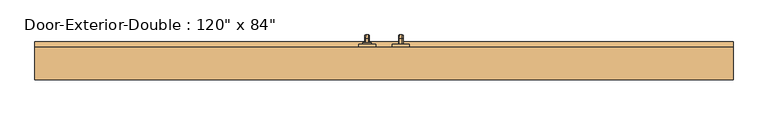
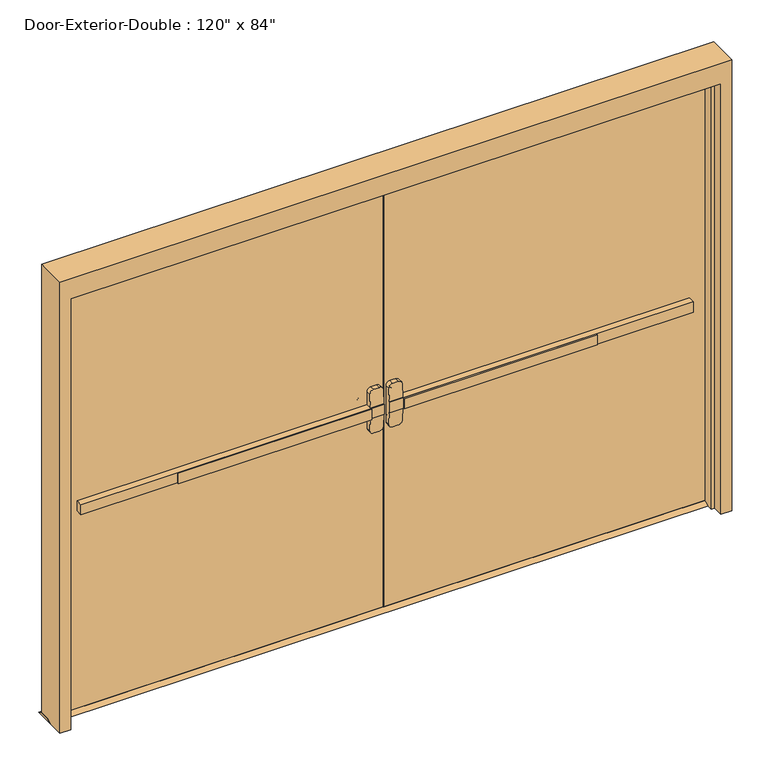
"""IFC4 building model written with IfcOpenShell, lengths in millimetres: door geometry."""

from ifc_helpers import new_model, si_unit, point, frame, frame_2d, origin, place, context, project, spatial, polyline, circle_curve, ellipse_curve, trimmed, segment, composite_curve, outline, extrude, faceted_brep, source, transform, mapped, element, save
from ifc_brep_helpers import plane_surface, cylinder_surface, revolved_surface, advanced_brep


def door_4e55e581(model_context):
    return source(origin(), model_context, "Body", "SolidModel", [
        extrude(outline(polyline([(-982.1333333, 0.0), (-982.1333333, 6.35), (-76.2, 6.35), (-76.2, 0.0), (-982.1333333, 0.0)])), frame((0.0, 0.0, 990.6), z_axis=(0.0, 0.0, 1.0), x_axis=(1.0, 0.0, 0.0)), (0.0, 0.0, 1.0), 50.8),
        advanced_brep(
        [(-12.7, 6.35, 1041.4), (-76.2, 6.35, 1041.4), (-1435.1, 6.35, 1041.4), (-1435.1, 6.35, 990.6), (-76.2, 6.35, 990.6), (-12.7, 6.35, 990.6), (-1435.1, 38.1, 1041.4), (-76.2, 38.1, 1041.4), (-76.2, 38.1, 1104.9), (-57.15, 38.1, 1123.95), (-31.75, 38.1, 1123.95), (-12.7, 38.1, 1104.9), (-12.7, 38.1, 927.1), (-31.75, 38.1, 908.05), (-57.15, 38.1, 908.05), (-76.2, 38.1, 927.1), (-76.2, 38.1, 990.6), (-1435.1, 38.1, 990.6), (-12.7, 9.5252467, 1041.4), (-76.2, 9.5252467, 1041.4), (-12.7, 9.5252467, 990.6), (-12.7, 14.5354269, 927.1), (-12.7, 14.5354269, 1104.9), (-76.2, 9.5252467, 990.6), (-76.2, 14.5354269, 1104.9), (-76.2, 14.5354269, 927.1), (-57.15, 16.038481, 1123.95), (-31.75, 16.038481, 1123.95), (-31.75, 16.038481, 908.05), (-57.15, 16.038481, 908.05)],
        [
            (0, 1),
            (1, 2),
            (2, 3),
            (3, 4),
            (4, 5),
            (5, 0),
            (6, 7),
            (7, 8),
            (8, 9, circle_curve(frame((-57.15, 38.1, 1104.9), z_axis=(0.0, 1.0, 0.0), x_axis=(-1.0, 0.0, 0.0)), 19.05)),
            (9, 10),
            (10, 11, circle_curve(frame((-31.75, 38.1, 1104.9), z_axis=(0.0, 1.0, 0.0), x_axis=(-1.0, 0.0, 0.0)), 19.05)),
            (11, 12),
            (12, 13, circle_curve(frame((-31.75, 38.1, 927.1), z_axis=(0.0, 1.0, 0.0), x_axis=(-1.0, 0.0, 0.0)), 19.05)),
            (13, 14),
            (14, 15, circle_curve(frame((-57.15, 38.1, 927.1), z_axis=(0.0, 1.0, 0.0), x_axis=(-1.0, 0.0, 0.0)), 19.05)),
            (15, 16),
            (16, 17),
            (17, 6),
            (0, 18),
            (18, 19),
            (19, 7),
            (6, 2),
            (5, 20),
            (20, 21),
            (21, 12),
            (11, 22),
            (22, 18),
            (16, 23),
            (23, 20),
            (3, 17),
            (19, 24),
            (24, 8),
            (15, 25),
            (25, 23),
            (9, 26),
            (26, 27),
            (27, 10),
            (13, 28),
            (28, 29),
            (29, 14),
            (29, 25, ellipse_curve(frame((-57.15, 14.5354269, 927.1), z_axis=(0.0, 0.9969018152893365, 0.07865602756830282), x_axis=(0.0, -0.07865602756830208, 0.9969018152893365)), 19.1092038, 19.05)),
            (24, 26, ellipse_curve(frame((-57.15, 14.5354269, 1104.9), z_axis=(0.0, 0.9969018152893376, -0.07865602756828934), x_axis=(0.0, -0.078656027568288, -0.9969018152893377)), 19.1092038, 19.05)),
            (27, 22, ellipse_curve(frame((-31.75, 14.5354269, 1104.9), z_axis=(0.0, 0.9969018152893376, -0.07865602756828934), x_axis=(0.0, -0.078656027568288, -0.9969018152893377)), 19.1092038, 19.05)),
            (21, 28, ellipse_curve(frame((-31.75, 14.5354269, 927.1), z_axis=(0.0, 0.9969018152893365, 0.07865602756830282), x_axis=(0.0, -0.07865602756830208, 0.9969018152893365)), 19.1092038, 19.05)),
        ],
        [
            plane_surface(frame((-12.7, 6.35, 1041.4), z_axis=(0.0, -1.0, 0.0), x_axis=(1.0, 0.0, 0.0))),
            plane_surface(frame((-12.7, 38.1, 1041.4), z_axis=(0.0, 1.0, 0.0), x_axis=(-1.0, 0.0, 0.0))),
            plane_surface(frame((-1435.1, 6.35, 1041.4), z_axis=(0.0, 0.0, 1.0), x_axis=(0.0, 1.0, 0.0))),
            plane_surface(frame((-12.7, 6.35, 1041.4), z_axis=(1.0, 0.0, 0.0), x_axis=(0.0, 1.0, 0.0))),
            plane_surface(frame((-12.7, 6.35, 990.6), z_axis=(0.0, 0.0, -1.0), x_axis=(0.0, 1.0, 0.0))),
            plane_surface(frame((-1435.1, 6.35, 990.6), z_axis=(-1.0, 0.0, 0.0), x_axis=(0.0, 1.0, 0.0))),
            plane_surface(frame((-76.2, 9.5252467, 927.1), z_axis=(-1.0, 0.0, 0.0), x_axis=(0.0, 1.0, 0.0))),
            plane_surface(frame((-57.15, 9.5252467, 1123.95), z_axis=(0.0, 0.0, 1.0), x_axis=(0.0, 1.0, 0.0))),
            plane_surface(frame((-31.75, 9.5252467, 908.05), z_axis=(0.0, 0.0, -1.0), x_axis=(0.0, 1.0, 0.0))),
            cylinder_surface(frame((-57.15, 38.1, 927.1), z_axis=(0.0, -1.0, 0.0), x_axis=(-1.0, 0.0, 0.0)), 19.05),
            cylinder_surface(frame((-57.15, 38.1, 1104.9), z_axis=(0.0, -1.0, 0.0), x_axis=(-1.0, 0.0, 0.0)), 19.05),
            cylinder_surface(frame((-31.75, 38.1, 1104.9), z_axis=(0.0, -1.0, 0.0), x_axis=(-1.0, 0.0, 0.0)), 19.05),
            cylinder_surface(frame((-31.75, 38.1, 927.1), z_axis=(0.0, -1.0, 0.0), x_axis=(-1.0, 0.0, 0.0)), 19.05),
            plane_surface(frame((-76.2, 9.5252467, 1041.4), z_axis=(0.0, -0.9969018152893376, 0.07865602756828934), x_axis=(1.0, 0.0, 0.0))),
            plane_surface(frame((-76.2, 16.038481, 908.05), z_axis=(0.0, -0.9969018152893365, -0.07865602756830282), x_axis=(1.0, 0.0, 0.0))),
        ],
        [
            (0, [[1, 2, 3, 4, 5, 6]]),
            (1, [[7, 8, 9, 10, 11, 12, 13, 14, 15, 16, 17, 18]]),
            (2, [[-2, -1, 19, 20, 21, -7, 22]]),
            (3, [[23, 24, 25, -12, 26, 27, -19, -6]]),
            (4, [[-17, 28, 29, -23, -5, -4, 30]]),
            (5, [[-22, -18, -30, -3]]),
            (6, [[-21, 31, 32, -8]]),
            (6, [[33, 34, -28, -16]]),
            (7, [[35, 36, 37, -10]]),
            (8, [[38, 39, 40, -14]]),
            (9, [[-40, 41, -33, -15]]),
            (10, [[-32, 42, -35, -9]]),
            (11, [[-37, 43, -26, -11]]),
            (12, [[-25, 44, -38, -13]]),
            (13, [[-27, -43, -36, -42, -31, -20]]),
            (14, [[-29, -34, -41, -39, -44, -24]]),
        ],
    ),
        extrude(outline(polyline([(82.55, 12.7), (107.95, 0.0), (12.7, 0.0), (38.1, 12.7), (82.55, 12.7)])), frame((-1574.8, 0.0, 0.0), z_axis=(1.0, 0.0, 0.0), x_axis=(0.0, 1.0, 0.0)), (0.0, 0.0, 1.0), 3149.6),
        extrude(outline(polyline([(982.1333333, 0.0), (76.2, 0.0), (76.2, 6.35), (982.1333333, 6.35), (982.1333333, 0.0)])), frame((0.0, 0.0, 990.6), z_axis=(0.0, 0.0, 1.0), x_axis=(1.0, 0.0, 0.0)), (0.0, 0.0, 1.0), 50.8),
        advanced_brep(
        [(12.7, 6.35, 1041.4), (12.7, 6.35, 990.6), (76.2, 6.35, 990.6), (1435.1, 6.35, 990.6), (1435.1, 6.35, 1041.4), (76.2, 6.35, 1041.4), (1435.1, 38.1, 1041.4), (1435.1, 38.1, 990.6), (76.2, 38.1, 990.6), (76.2, 38.1, 927.1), (57.15, 38.1, 908.05), (31.75, 38.1, 908.05), (12.7, 38.1, 927.1), (12.7, 38.1, 1104.9), (31.75, 38.1, 1123.95), (57.15, 38.1, 1123.95), (76.2, 38.1, 1104.9), (76.2, 38.1, 1041.4), (76.2, 9.5252467, 1041.4), (12.7, 9.5252467, 1041.4), (12.7, 14.5354269, 1104.9), (12.7, 14.5354269, 927.1), (12.7, 9.5252467, 990.6), (76.2, 9.5252467, 990.6), (76.2, 14.5354269, 927.1), (76.2, 14.5354269, 1104.9), (31.75, 16.038481, 1123.95), (57.15, 16.038481, 1123.95), (57.15, 16.038481, 908.05), (31.75, 16.038481, 908.05)],
        [
            (0, 1),
            (1, 2),
            (2, 3),
            (3, 4),
            (4, 5),
            (5, 0),
            (6, 7),
            (7, 8),
            (8, 9),
            (9, 10, circle_curve(frame((57.15, 38.1, 927.1), z_axis=(0.0, 1.0, 0.0), x_axis=(1.0, 0.0, 0.0)), 19.05)),
            (10, 11),
            (11, 12, circle_curve(frame((31.75, 38.1, 927.1), z_axis=(0.0, 1.0, 0.0), x_axis=(1.0, 0.0, 0.0)), 19.05)),
            (12, 13),
            (13, 14, circle_curve(frame((31.75, 38.1, 1104.9), z_axis=(0.0, 1.0, 0.0), x_axis=(1.0, 0.0, 0.0)), 19.05)),
            (14, 15),
            (15, 16, circle_curve(frame((57.15, 38.1, 1104.9), z_axis=(0.0, 1.0, 0.0), x_axis=(1.0, 0.0, 0.0)), 19.05)),
            (16, 17),
            (17, 6),
            (4, 6),
            (17, 18),
            (18, 19),
            (19, 0),
            (19, 20),
            (20, 13),
            (12, 21),
            (21, 22),
            (22, 1),
            (7, 3),
            (22, 23),
            (23, 8),
            (23, 24),
            (24, 9),
            (16, 25),
            (25, 18),
            (14, 26),
            (26, 27),
            (27, 15),
            (10, 28),
            (28, 29),
            (29, 11),
            (24, 28, ellipse_curve(frame((57.15, 14.5354269, 927.1), z_axis=(0.0, 0.9969018152893365, 0.07865602756830282), x_axis=(0.0, -0.07865602756830208, 0.9969018152893365)), 19.1092038, 19.05)),
            (27, 25, ellipse_curve(frame((57.15, 14.5354269, 1104.9), z_axis=(0.0, 0.9969018152893376, -0.07865602756828934), x_axis=(0.0, -0.078656027568288, -0.9969018152893377)), 19.1092038, 19.05)),
            (20, 26, ellipse_curve(frame((31.75, 14.5354269, 1104.9), z_axis=(0.0, 0.9969018152893376, -0.07865602756828934), x_axis=(0.0, -0.078656027568288, -0.9969018152893377)), 19.1092038, 19.05)),
            (29, 21, ellipse_curve(frame((31.75, 14.5354269, 927.1), z_axis=(0.0, 0.9969018152893365, 0.07865602756830282), x_axis=(0.0, -0.07865602756830208, 0.9969018152893365)), 19.1092038, 19.05)),
        ],
        [
            plane_surface(frame((12.7, 6.35, 1041.4), z_axis=(0.0, -1.0, 0.0), x_axis=(-1.0, 0.0, 0.0))),
            plane_surface(frame((12.7, 38.1, 1041.4), z_axis=(0.0, 1.0, 0.0), x_axis=(1.0, 0.0, 0.0))),
            plane_surface(frame((1435.1, 6.35, 1041.4), z_axis=(0.0, 0.0, 1.0), x_axis=(0.0, 1.0, 0.0))),
            plane_surface(frame((12.7, 6.35, 1041.4), z_axis=(-1.0, 0.0, 0.0), x_axis=(0.0, 1.0, 0.0))),
            plane_surface(frame((12.7, 6.35, 990.6), z_axis=(0.0, 0.0, -1.0), x_axis=(0.0, 1.0, 0.0))),
            plane_surface(frame((1435.1, 6.35, 990.6), z_axis=(1.0, 0.0, 0.0), x_axis=(0.0, 1.0, 0.0))),
            plane_surface(frame((76.2, 9.5252467, 927.1), z_axis=(1.0, 0.0, 0.0), x_axis=(0.0, 1.0, 0.0))),
            plane_surface(frame((57.15, 9.5252467, 1123.95), z_axis=(0.0, 0.0, 1.0), x_axis=(0.0, 1.0, 0.0))),
            plane_surface(frame((31.75, 9.5252467, 908.05), z_axis=(0.0, 0.0, -1.0), x_axis=(0.0, 1.0, 0.0))),
            cylinder_surface(frame((57.15, 38.1, 927.1), z_axis=(0.0, -1.0, 0.0), x_axis=(1.0, 0.0, 0.0)), 19.05),
            cylinder_surface(frame((57.15, 38.1, 1104.9), z_axis=(0.0, -1.0, 0.0), x_axis=(1.0, 0.0, 0.0)), 19.05),
            cylinder_surface(frame((31.75, 38.1, 1104.9), z_axis=(0.0, -1.0, 0.0), x_axis=(1.0, 0.0, 0.0)), 19.05),
            cylinder_surface(frame((31.75, 38.1, 927.1), z_axis=(0.0, -1.0, 0.0), x_axis=(1.0, 0.0, 0.0)), 19.05),
            plane_surface(frame((76.2, 9.5252467, 1041.4), z_axis=(0.0, -0.9969018152893376, 0.07865602756828934), x_axis=(-1.0, 0.0, 0.0))),
            plane_surface(frame((76.2, 16.038481, 908.05), z_axis=(0.0, -0.9969018152893365, -0.07865602756830282), x_axis=(-1.0, 0.0, 0.0))),
        ],
        [
            (0, [[1, 2, 3, 4, 5, 6]]),
            (1, [[7, 8, 9, 10, 11, 12, 13, 14, 15, 16, 17, 18]]),
            (2, [[19, -18, 20, 21, 22, -6, -5]]),
            (3, [[-1, -22, 23, 24, -13, 25, 26, 27]]),
            (4, [[28, -3, -2, -27, 29, 30, -8]]),
            (5, [[-4, -28, -7, -19]]),
            (6, [[-9, -30, 31, 32]]),
            (6, [[-17, 33, 34, -20]]),
            (7, [[-15, 35, 36, 37]]),
            (8, [[-11, 38, 39, 40]]),
            (9, [[-10, -32, 41, -38]]),
            (10, [[-16, -37, 42, -33]]),
            (11, [[-14, -24, 43, -35]]),
            (12, [[-12, -40, 44, -25]]),
            (13, [[-21, -34, -42, -36, -43, -23]]),
            (14, [[-26, -44, -39, -41, -31, -29]]),
        ],
    ),
        advanced_brep(
        [(66.2, 95.25, 1017.190625), (66.2, 95.25, 1014.809375), (69.771875, 95.25, 1011.2375), (82.6284594, 95.25, 1011.2375), (86.2, 95.25, 1014.8090406), (86.2, 95.25, 1017.190625), (82.628125, 95.25, 1020.7625), (69.771875, 95.25, 1020.7625), (66.2, 95.25, 887.809375), (69.771875, 95.25, 884.2375), (82.628125, 95.25, 884.2375), (86.2, 95.25, 887.809375), (86.2, 95.25, 890.1909594), (82.6284594, 95.25, 893.7625), (69.771875, 95.25, 893.7625), (66.2, 95.25, 890.190625), (66.2, 120.65, 1017.190625), (66.2, 134.540625, 1003.3), (66.2, 134.540625, 901.7), (66.2, 120.65, 887.809375), (66.2, 120.65, 890.190625), (66.2, 132.159375, 901.7), (66.2, 132.159375, 1003.3), (66.2, 120.65, 1014.809375), (69.771875, 120.65, 1011.2375), (82.6284594, 120.65, 1011.2375), (86.2, 120.65, 1014.8090406), (86.2, 132.1590406, 1003.3), (86.2, 132.1590406, 901.7), (86.2, 120.65, 890.1909594), (86.2, 120.65, 887.809375), (86.2, 134.540625, 901.7), (86.2, 134.540625, 1003.3), (86.2, 120.65, 1017.190625), (82.628125, 120.65, 1020.7625), (69.771875, 120.65, 1020.7625), (69.771875, 128.5875, 1003.3), (82.6284594, 128.5875, 1003.3), (82.628125, 138.1125, 1003.3), (69.771875, 138.1125, 1003.3), (69.771875, 128.5875, 901.7), (82.6284594, 128.5875, 901.7), (82.628125, 138.1125, 901.7), (69.771875, 138.1125, 901.7), (69.771875, 120.65, 893.7625), (82.6284594, 120.65, 893.7625), (82.628125, 120.65, 884.2375), (69.771875, 120.65, 884.2375)],
        [
            (0, 1),
            (1, 2, circle_curve(frame((69.771875, 95.25, 1014.809375), z_axis=(0.0, -1.0, 0.0), x_axis=(0.0, 0.0, 1.0)), 3.571875)),
            (2, 3),
            (3, 4, circle_curve(frame((82.6284594, 95.25, 1014.8090406), z_axis=(0.0, -1.0, 0.0), x_axis=(0.0, 0.0, 1.0)), 3.5715406)),
            (4, 5),
            (5, 6, circle_curve(frame((82.628125, 95.25, 1017.190625), z_axis=(0.0, -1.0, 0.0), x_axis=(0.0, 0.0, 1.0)), 3.571875)),
            (6, 7),
            (7, 0, circle_curve(frame((69.771875, 95.25, 1017.190625), z_axis=(0.0, -1.0, 0.0), x_axis=(0.0, 0.0, 1.0)), 3.571875)),
            (8, 9, circle_curve(frame((69.771875, 95.25, 887.809375), z_axis=(0.0, -1.0, 0.0), x_axis=(0.0, 0.0, -1.0)), 3.571875)),
            (9, 10),
            (10, 11, circle_curve(frame((82.628125, 95.25, 887.809375), z_axis=(0.0, -1.0, 0.0), x_axis=(0.0, 0.0, -1.0)), 3.571875)),
            (11, 12),
            (12, 13, circle_curve(frame((82.6284594, 95.25, 890.1909594), z_axis=(0.0, -1.0, 0.0), x_axis=(0.0, 0.0, -1.0)), 3.5715406)),
            (13, 14),
            (14, 15, circle_curve(frame((69.771875, 95.25, 890.190625), z_axis=(0.0, -1.0, 0.0), x_axis=(0.0, 0.0, -1.0)), 3.571875)),
            (15, 8),
            (0, 16),
            (16, 17, circle_curve(frame((66.2, 120.65, 1003.3), z_axis=(-1.0, 0.0, 0.0), x_axis=(0.0, 0.0, 1.0)), 13.890625)),
            (17, 18),
            (18, 19, circle_curve(frame((66.2, 120.65, 901.7), z_axis=(-1.0, 0.0, 0.0), x_axis=(0.0, 1.0, 0.0)), 13.890625)),
            (19, 8),
            (15, 20),
            (20, 21, circle_curve(frame((66.2, 120.65, 901.7), z_axis=(1.0, 0.0, 0.0), x_axis=(0.0, 1.0, 0.0)), 11.509375)),
            (21, 22),
            (22, 23, circle_curve(frame((66.2, 120.65, 1003.3), z_axis=(1.0, 0.0, 0.0), x_axis=(0.0, 0.0, 1.0)), 11.509375)),
            (23, 1),
            (23, 24, circle_curve(frame((69.771875, 120.65, 1014.809375), z_axis=(0.0, -1.0, 0.0), x_axis=(0.0, 0.0, 1.0)), 3.571875)),
            (24, 2),
            (24, 25),
            (25, 3),
            (25, 26, circle_curve(frame((82.6284594, 120.65, 1014.8090406), z_axis=(0.0, -1.0, 0.0), x_axis=(0.0, 0.0, 1.0)), 3.5715406)),
            (26, 4),
            (26, 27, circle_curve(frame((86.2, 120.65, 1003.3), z_axis=(-1.0, 0.0, 0.0), x_axis=(0.0, 0.0, 1.0)), 11.5090406)),
            (27, 28),
            (28, 29, circle_curve(frame((86.2, 120.65, 901.7), z_axis=(-1.0, 0.0, 0.0), x_axis=(0.0, 1.0, 0.0)), 11.5090406)),
            (29, 12),
            (11, 30),
            (30, 31, circle_curve(frame((86.2, 120.65, 901.7), z_axis=(1.0, 0.0, 0.0), x_axis=(0.0, 1.0, 0.0)), 13.890625)),
            (31, 32),
            (32, 33, circle_curve(frame((86.2, 120.65, 1003.3), z_axis=(1.0, 0.0, 0.0), x_axis=(0.0, 0.0, 1.0)), 13.890625)),
            (33, 5),
            (33, 34, circle_curve(frame((82.628125, 120.65, 1017.190625), z_axis=(0.0, -1.0, 0.0), x_axis=(0.0, 0.0, 1.0)), 3.571875)),
            (34, 6),
            (34, 35),
            (35, 7),
            (35, 16, circle_curve(frame((69.771875, 120.65, 1017.190625), z_axis=(0.0, -1.0, 0.0), x_axis=(0.0, 0.0, 1.0)), 3.571875)),
            (36, 24, circle_curve(frame((69.771875, 120.65, 1003.3), z_axis=(1.0, 0.0, 0.0), x_axis=(0.0, 0.0, 1.0)), 7.9375)),
            (22, 36, circle_curve(frame((69.771875, 132.159375, 1003.3), z_axis=(0.0, 0.0, 1.0), x_axis=(0.0, 1.0, 0.0)), 3.571875)),
            (37, 25, circle_curve(frame((82.6284594, 120.65, 1003.3), z_axis=(1.0, 0.0, 0.0), x_axis=(0.0, 0.0, 1.0)), 7.9375)),
            (36, 37),
            (37, 27, circle_curve(frame((82.6284594, 132.1590406, 1003.3), z_axis=(0.0, 0.0, 1.0), x_axis=(0.0, 1.0, 0.0)), 3.5715406)),
            (38, 34, circle_curve(frame((82.628125, 120.65, 1003.3), z_axis=(1.0, 0.0, 0.0), x_axis=(0.0, 0.0, 1.0)), 17.4625)),
            (32, 38, circle_curve(frame((82.628125, 134.540625, 1003.3), z_axis=(0.0, 0.0, 1.0), x_axis=(0.0, 1.0, 0.0)), 3.571875)),
            (39, 35, circle_curve(frame((69.771875, 120.65, 1003.3), z_axis=(1.0, 0.0, 0.0), x_axis=(0.0, 0.0, 1.0)), 17.4625)),
            (38, 39),
            (39, 17, circle_curve(frame((69.771875, 134.540625, 1003.3), z_axis=(0.0, 0.0, 1.0), x_axis=(0.0, 1.0, 0.0)), 3.571875)),
            (21, 40, circle_curve(frame((69.771875, 132.159375, 901.7), z_axis=(0.0, 0.0, 1.0), x_axis=(0.0, 1.0, 0.0)), 3.571875)),
            (40, 36),
            (40, 41),
            (41, 37),
            (41, 28, circle_curve(frame((82.6284594, 132.1590406, 901.7), z_axis=(0.0, 0.0, 1.0), x_axis=(0.0, 1.0, 0.0)), 3.5715406)),
            (31, 42, circle_curve(frame((82.628125, 134.540625, 901.7), z_axis=(0.0, 0.0, 1.0), x_axis=(0.0, 1.0, 0.0)), 3.571875)),
            (42, 38),
            (42, 43),
            (43, 39),
            (43, 18, circle_curve(frame((69.771875, 134.540625, 901.7), z_axis=(0.0, 0.0, 1.0), x_axis=(0.0, 1.0, 0.0)), 3.571875)),
            (44, 40, circle_curve(frame((69.771875, 120.65, 901.7), z_axis=(1.0, 0.0, 0.0), x_axis=(0.0, 1.0, 0.0)), 7.9375)),
            (20, 44, circle_curve(frame((69.771875, 120.65, 890.190625), z_axis=(0.0, 1.0, 0.0), x_axis=(0.0, 0.0, -1.0)), 3.571875)),
            (45, 41, circle_curve(frame((82.6284594, 120.65, 901.7), z_axis=(1.0, 0.0, 0.0), x_axis=(0.0, 1.0, 0.0)), 7.9375)),
            (44, 45),
            (45, 29, circle_curve(frame((82.6284594, 120.65, 890.1909594), z_axis=(0.0, 1.0, 0.0), x_axis=(0.0, 0.0, -1.0)), 3.5715406)),
            (46, 42, circle_curve(frame((82.628125, 120.65, 901.7), z_axis=(1.0, 0.0, 0.0), x_axis=(0.0, 1.0, 0.0)), 17.4625)),
            (30, 46, circle_curve(frame((82.628125, 120.65, 887.809375), z_axis=(0.0, 1.0, 0.0), x_axis=(0.0, 0.0, -1.0)), 3.571875)),
            (47, 43, circle_curve(frame((69.771875, 120.65, 901.7), z_axis=(1.0, 0.0, 0.0), x_axis=(0.0, 1.0, 0.0)), 17.4625)),
            (46, 47),
            (47, 19, circle_curve(frame((69.771875, 120.65, 887.809375), z_axis=(0.0, 1.0, 0.0), x_axis=(0.0, 0.0, -1.0)), 3.571875)),
            (14, 44),
            (13, 45),
            (10, 46),
            (9, 47),
        ],
        [
            plane_surface(frame((76.2, 95.25, 1016.0), z_axis=(0.0, -1.0, 0.0), x_axis=(1.0, 0.0, 0.0))),
            plane_surface(frame((76.2, 95.25, 889.0), z_axis=(0.0, -1.0, 0.0), x_axis=(1.0, 0.0, 0.0))),
            plane_surface(frame((66.2, 95.25, 1017.190625), z_axis=(-1.0, 0.0, 0.0), x_axis=(0.0, 1.0, 0.0))),
            cylinder_surface(frame((69.771875, 95.25, 1014.809375), z_axis=(0.0, -1.0, 0.0), x_axis=(0.0, 0.0, 1.0)), 3.571875),
            plane_surface(frame((69.771875, 95.25, 1011.2375), z_axis=(0.0, 0.0, -1.0), x_axis=(0.0, 1.0, 0.0))),
            cylinder_surface(frame((82.6284594, 95.25, 1014.8090406), z_axis=(0.0, -1.0, 0.0), x_axis=(0.0, 0.0, 1.0)), 3.5715406),
            plane_surface(frame((86.2, 95.25, 1014.8090406), z_axis=(1.0, 0.0, 0.0), x_axis=(0.0, 1.0, 0.0))),
            cylinder_surface(frame((82.628125, 95.25, 1017.190625), z_axis=(0.0, -1.0, 0.0), x_axis=(0.0, 0.0, 1.0)), 3.571875),
            plane_surface(frame((82.628125, 95.25, 1020.7625), z_axis=(0.0, 0.0, 1.0), x_axis=(0.0, 1.0, 0.0))),
            cylinder_surface(frame((69.771875, 95.25, 1017.190625), z_axis=(0.0, -1.0, 0.0), x_axis=(0.0, 0.0, 1.0)), 3.571875),
            revolved_surface(trimmed(ellipse_curve(frame((69.771875, 120.65, 1014.809375), z_axis=(0.0, -1.0, 0.0), x_axis=(0.0, 0.0, 1.0)), 3.571875, 3.571875), [point((66.2, 120.65, 1014.809375))], [point((69.771875, 120.65, 1011.2375))], True, "CARTESIAN"), (76.2, 120.65, 1003.3), (-1.0, 0.0, 0.0)),
            revolved_surface(polyline([(69.771875, 120.65, 1011.2375), (82.6284594, 120.65, 1011.2375)]), (76.2, 120.65, 1003.3), (-1.0, 0.0, 0.0)),
            revolved_surface(trimmed(ellipse_curve(frame((82.6284594, 120.65, 1014.8090406), z_axis=(0.0, -1.0, 0.0), x_axis=(0.0, 0.0, 1.0)), 3.5715406, 3.5715406), [point((82.6284594, 120.65, 1011.2375))], [point((86.2, 120.65, 1014.8090406))], True, "CARTESIAN"), (76.2, 120.65, 1003.3), (-1.0, 0.0, 0.0)),
            revolved_surface(trimmed(ellipse_curve(frame((82.628125, 120.65, 1017.190625), z_axis=(0.0, -1.0, 0.0), x_axis=(0.0, 0.0, 1.0)), 3.571875, 3.571875), [point((86.2, 120.65, 1017.190625))], [point((82.628125, 120.65, 1020.7625))], True, "CARTESIAN"), (76.2, 120.65, 1003.3), (-1.0, 0.0, 0.0)),
            cylinder_surface(frame((76.2, 120.65, 1003.3), z_axis=(-1.0, 0.0, 0.0), x_axis=(0.0, 0.0, 1.0)), 17.4625),
            revolved_surface(trimmed(ellipse_curve(frame((69.771875, 120.65, 1017.190625), z_axis=(0.0, -1.0, 0.0), x_axis=(0.0, 0.0, 1.0)), 3.571875, 3.571875), [point((69.771875, 120.65, 1020.7625))], [point((66.2, 120.65, 1017.190625))], True, "CARTESIAN"), (76.2, 120.65, 1003.3), (-1.0, 0.0, 0.0)),
            cylinder_surface(frame((69.771875, 132.159375, 1003.3), z_axis=(0.0, 0.0, 1.0), x_axis=(0.0, 1.0, 0.0)), 3.571875),
            plane_surface(frame((69.771875, 128.5875, 1003.3), z_axis=(0.0, -1.0, 0.0), x_axis=(0.0, 0.0, -1.0))),
            cylinder_surface(frame((82.6284594, 132.1590406, 1003.3), z_axis=(0.0, 0.0, 1.0), x_axis=(0.0, 1.0, 0.0)), 3.5715406),
            cylinder_surface(frame((82.628125, 134.540625, 1003.3), z_axis=(0.0, 0.0, 1.0), x_axis=(0.0, 1.0, 0.0)), 3.571875),
            plane_surface(frame((82.628125, 138.1125, 1003.3), z_axis=(0.0, 1.0, 0.0), x_axis=(0.0, 0.0, -1.0))),
            cylinder_surface(frame((69.771875, 134.540625, 1003.3), z_axis=(0.0, 0.0, 1.0), x_axis=(0.0, 1.0, 0.0)), 3.571875),
            revolved_surface(trimmed(ellipse_curve(frame((69.771875, 132.159375, 901.7), z_axis=(0.0, 0.0, 1.0), x_axis=(0.0, 1.0, 0.0)), 3.571875, 3.571875), [point((66.2, 132.159375, 901.7))], [point((69.771875, 128.5875, 901.7))], True, "CARTESIAN"), (76.2, 120.65, 901.7), (-1.0, 0.0, 0.0)),
            revolved_surface(polyline([(69.771875, 128.5875, 901.7), (82.6284594, 128.5875, 901.7)]), (76.2, 120.65, 901.7), (-1.0, 0.0, 0.0)),
            revolved_surface(trimmed(ellipse_curve(frame((82.6284594, 132.1590406, 901.7), z_axis=(0.0, 0.0, 1.0), x_axis=(0.0, 1.0, 0.0)), 3.5715406, 3.5715406), [point((82.6284594, 128.5875, 901.7))], [point((86.2, 132.1590406, 901.7))], True, "CARTESIAN"), (76.2, 120.65, 901.7), (-1.0, 0.0, 0.0)),
            revolved_surface(trimmed(ellipse_curve(frame((82.628125, 134.540625, 901.7), z_axis=(0.0, 0.0, 1.0), x_axis=(0.0, 1.0, 0.0)), 3.571875, 3.571875), [point((86.2, 134.540625, 901.7))], [point((82.628125, 138.1125, 901.7))], True, "CARTESIAN"), (76.2, 120.65, 901.7), (-1.0, 0.0, 0.0)),
            cylinder_surface(frame((76.2, 120.65, 901.7), z_axis=(-1.0, 0.0, 0.0), x_axis=(0.0, 1.0, 0.0)), 17.4625),
            revolved_surface(trimmed(ellipse_curve(frame((69.771875, 134.540625, 901.7), z_axis=(0.0, 0.0, 1.0), x_axis=(0.0, 1.0, 0.0)), 3.571875, 3.571875), [point((69.771875, 138.1125, 901.7))], [point((66.2, 134.540625, 901.7))], True, "CARTESIAN"), (76.2, 120.65, 901.7), (-1.0, 0.0, 0.0)),
            cylinder_surface(frame((69.771875, 120.65, 890.190625), z_axis=(0.0, 1.0, 0.0), x_axis=(0.0, 0.0, -1.0)), 3.571875),
            plane_surface(frame((69.771875, 120.65, 893.7625), z_axis=(0.0, 0.0, 1.0), x_axis=(0.0, -1.0, 0.0))),
            cylinder_surface(frame((82.6284594, 120.65, 890.1909594), z_axis=(0.0, 1.0, 0.0), x_axis=(0.0, 0.0, -1.0)), 3.5715406),
            cylinder_surface(frame((82.628125, 120.65, 887.809375), z_axis=(0.0, 1.0, 0.0), x_axis=(0.0, 0.0, -1.0)), 3.571875),
            plane_surface(frame((82.628125, 120.65, 884.2375), z_axis=(0.0, 0.0, -1.0), x_axis=(0.0, -1.0, 0.0))),
            cylinder_surface(frame((69.771875, 120.65, 887.809375), z_axis=(0.0, 1.0, 0.0), x_axis=(0.0, 0.0, -1.0)), 3.571875),
        ],
        [
            (0, [[1, 2, 3, 4, 5, 6, 7, 8]]),
            (1, [[9, 10, 11, 12, 13, 14, 15, 16]]),
            (2, [[-1, 17, 18, 19, 20, 21, -16, 22, 23, 24, 25, 26]]),
            (3, [[-2, -26, 27, 28]]),
            (4, [[-3, -28, 29, 30]]),
            (5, [[-4, -30, 31, 32]]),
            (6, [[-5, -32, 33, 34, 35, 36, -12, 37, 38, 39, 40, 41]]),
            (7, [[-6, -41, 42, 43]]),
            (8, [[-7, -43, 44, 45]]),
            (9, [[-8, -45, 46, -17]]),
            (10, [[47, -27, -25, 48]]),
            (11, [[49, -29, -47, 50]]),
            (12, [[-33, -31, -49, 51]]),
            (13, [[52, -42, -40, 53]]),
            (14, [[54, -44, -52, 55]]),
            (15, [[-18, -46, -54, 56]]),
            (16, [[-48, -24, 57, 58]]),
            (17, [[-50, -58, 59, 60]]),
            (18, [[-51, -60, 61, -34]]),
            (19, [[-53, -39, 62, 63]]),
            (20, [[-55, -63, 64, 65]]),
            (21, [[-56, -65, 66, -19]]),
            (22, [[67, -57, -23, 68]]),
            (23, [[69, -59, -67, 70]]),
            (24, [[-35, -61, -69, 71]]),
            (25, [[72, -62, -38, 73]]),
            (26, [[74, -64, -72, 75]]),
            (27, [[-20, -66, -74, 76]]),
            (28, [[-68, -22, -15, 77]]),
            (29, [[-70, -77, -14, 78]]),
            (30, [[-71, -78, -13, -36]]),
            (31, [[-73, -37, -11, 79]]),
            (32, [[-75, -79, -10, 80]]),
            (33, [[-76, -80, -9, -21]]),
        ],
    ),
        extrude(outline(composite_curve([segment(trimmed(circle_curve(frame_2d((1113.0338574, 76.2)), 89.3016225), [point((1193.8, 114.3))], [point((1193.8, 38.1))], False, "CARTESIAN"), True, "CONTINUOUS"), segment(polyline([(1193.8, 38.1), (838.2, 38.1)]), True, "CONTINUOUS"), segment(trimmed(circle_curve(frame_2d((918.9661426, 76.2)), 89.3016225), [point((838.2, 38.1))], [point((838.2, 114.3))], False, "CARTESIAN"), True, "CONTINUOUS"), segment(polyline([(838.2, 114.3), (1193.8, 114.3)]), True, "CONTINUOUS")], self_intersect=False)), frame((0.0, 82.55, 0.0), z_axis=(0.0, 1.0, 0.0), x_axis=(0.0, 0.0, 1.0)), (0.0, 0.0, 1.0), 12.7),
        advanced_brep(
        [(-86.2, 95.25, 1017.190625), (-86.2, 95.25, 1014.809375), (-82.628125, 95.25, 1011.2375), (-69.7715406, 95.25, 1011.2375), (-66.2, 95.25, 1014.8090406), (-66.2, 95.25, 1017.190625), (-69.771875, 95.25, 1020.7625), (-82.628125, 95.25, 1020.7625), (-86.2, 95.25, 887.809375), (-82.628125, 95.25, 884.2375), (-69.771875, 95.25, 884.2375), (-66.2, 95.25, 887.809375), (-66.2, 95.25, 890.1909594), (-69.7715406, 95.25, 893.7625), (-82.628125, 95.25, 893.7625), (-86.2, 95.25, 890.190625), (-86.2, 120.65, 1017.190625), (-86.2, 134.540625, 1003.3), (-86.2, 134.540625, 901.7), (-86.2, 120.65, 887.809375), (-86.2, 120.65, 890.190625), (-86.2, 132.159375, 901.7), (-86.2, 132.159375, 1003.3), (-86.2, 120.65, 1014.809375), (-82.628125, 120.65, 1011.2375), (-69.7715406, 120.65, 1011.2375), (-66.2, 120.65, 1014.8090406), (-66.2, 132.1590406, 1003.3), (-66.2, 132.1590406, 901.7), (-66.2, 120.65, 890.1909594), (-66.2, 120.65, 887.809375), (-66.2, 134.540625, 901.7), (-66.2, 134.540625, 1003.3), (-66.2, 120.65, 1017.190625), (-69.771875, 120.65, 1020.7625), (-82.628125, 120.65, 1020.7625), (-82.628125, 128.5875, 1003.3), (-69.7715406, 128.5875, 1003.3), (-69.771875, 138.1125, 1003.3), (-82.628125, 138.1125, 1003.3), (-82.628125, 128.5875, 901.7), (-69.7715406, 128.5875, 901.7), (-69.771875, 138.1125, 901.7), (-82.628125, 138.1125, 901.7), (-82.628125, 120.65, 893.7625), (-69.7715406, 120.65, 893.7625), (-69.771875, 120.65, 884.2375), (-82.628125, 120.65, 884.2375)],
        [
            (0, 1),
            (1, 2, circle_curve(frame((-82.628125, 95.25, 1014.809375), z_axis=(0.0, -1.0, 0.0), x_axis=(0.0, 0.0, 1.0)), 3.571875)),
            (2, 3),
            (3, 4, circle_curve(frame((-69.7715406, 95.25, 1014.8090406), z_axis=(0.0, -1.0, 0.0), x_axis=(0.0, 0.0, 1.0)), 3.5715406)),
            (4, 5),
            (5, 6, circle_curve(frame((-69.771875, 95.25, 1017.190625), z_axis=(0.0, -1.0, 0.0), x_axis=(0.0, 0.0, 1.0)), 3.571875)),
            (6, 7),
            (7, 0, circle_curve(frame((-82.628125, 95.25, 1017.190625), z_axis=(0.0, -1.0, 0.0), x_axis=(0.0, 0.0, 1.0)), 3.571875)),
            (8, 9, circle_curve(frame((-82.628125, 95.25, 887.809375), z_axis=(0.0, -1.0, 0.0), x_axis=(0.0, 0.0, -1.0)), 3.571875)),
            (9, 10),
            (10, 11, circle_curve(frame((-69.771875, 95.25, 887.809375), z_axis=(0.0, -1.0, 0.0), x_axis=(0.0, 0.0, -1.0)), 3.571875)),
            (11, 12),
            (12, 13, circle_curve(frame((-69.7715406, 95.25, 890.1909594), z_axis=(0.0, -1.0, 0.0), x_axis=(0.0, 0.0, -1.0)), 3.5715406)),
            (13, 14),
            (14, 15, circle_curve(frame((-82.628125, 95.25, 890.190625), z_axis=(0.0, -1.0, 0.0), x_axis=(0.0, 0.0, -1.0)), 3.571875)),
            (15, 8),
            (0, 16),
            (16, 17, circle_curve(frame((-86.2, 120.65, 1003.3), z_axis=(-1.0, 0.0, 0.0), x_axis=(0.0, 0.0, 1.0)), 13.890625)),
            (17, 18),
            (18, 19, circle_curve(frame((-86.2, 120.65, 901.7), z_axis=(-1.0, 0.0, 0.0), x_axis=(0.0, 1.0, 0.0)), 13.890625)),
            (19, 8),
            (15, 20),
            (20, 21, circle_curve(frame((-86.2, 120.65, 901.7), z_axis=(1.0, 0.0, 0.0), x_axis=(0.0, 1.0, 0.0)), 11.509375)),
            (21, 22),
            (22, 23, circle_curve(frame((-86.2, 120.65, 1003.3), z_axis=(1.0, 0.0, 0.0), x_axis=(0.0, 0.0, 1.0)), 11.509375)),
            (23, 1),
            (23, 24, circle_curve(frame((-82.628125, 120.65, 1014.809375), z_axis=(0.0, -1.0, 0.0), x_axis=(0.0, 0.0, 1.0)), 3.571875)),
            (24, 2),
            (24, 25),
            (25, 3),
            (25, 26, circle_curve(frame((-69.7715406, 120.65, 1014.8090406), z_axis=(0.0, -1.0, 0.0), x_axis=(0.0, 0.0, 1.0)), 3.5715406)),
            (26, 4),
            (26, 27, circle_curve(frame((-66.2, 120.65, 1003.3), z_axis=(-1.0, 0.0, 0.0), x_axis=(0.0, 0.0, 1.0)), 11.5090406)),
            (27, 28),
            (28, 29, circle_curve(frame((-66.2, 120.65, 901.7), z_axis=(-1.0, 0.0, 0.0), x_axis=(0.0, 1.0, 0.0)), 11.5090406)),
            (29, 12),
            (11, 30),
            (30, 31, circle_curve(frame((-66.2, 120.65, 901.7), z_axis=(1.0, 0.0, 0.0), x_axis=(0.0, 1.0, 0.0)), 13.890625)),
            (31, 32),
            (32, 33, circle_curve(frame((-66.2, 120.65, 1003.3), z_axis=(1.0, 0.0, 0.0), x_axis=(0.0, 0.0, 1.0)), 13.890625)),
            (33, 5),
            (33, 34, circle_curve(frame((-69.771875, 120.65, 1017.190625), z_axis=(0.0, -1.0, 0.0), x_axis=(0.0, 0.0, 1.0)), 3.571875)),
            (34, 6),
            (34, 35),
            (35, 7),
            (35, 16, circle_curve(frame((-82.628125, 120.65, 1017.190625), z_axis=(0.0, -1.0, 0.0), x_axis=(0.0, 0.0, 1.0)), 3.571875)),
            (36, 24, circle_curve(frame((-82.628125, 120.65, 1003.3), z_axis=(1.0, 0.0, 0.0), x_axis=(0.0, 0.0, 1.0)), 7.9375)),
            (22, 36, circle_curve(frame((-82.628125, 132.159375, 1003.3), z_axis=(0.0, 0.0, 1.0), x_axis=(0.0, 1.0, 0.0)), 3.571875)),
            (37, 25, circle_curve(frame((-69.7715406, 120.65, 1003.3), z_axis=(1.0, 0.0, 0.0), x_axis=(0.0, 0.0, 1.0)), 7.9375)),
            (36, 37),
            (37, 27, circle_curve(frame((-69.7715406, 132.1590406, 1003.3), z_axis=(0.0, 0.0, 1.0), x_axis=(0.0, 1.0, 0.0)), 3.5715406)),
            (38, 34, circle_curve(frame((-69.771875, 120.65, 1003.3), z_axis=(1.0, 0.0, 0.0), x_axis=(0.0, 0.0, 1.0)), 17.4625)),
            (32, 38, circle_curve(frame((-69.771875, 134.540625, 1003.3), z_axis=(0.0, 0.0, 1.0), x_axis=(0.0, 1.0, 0.0)), 3.571875)),
            (39, 35, circle_curve(frame((-82.628125, 120.65, 1003.3), z_axis=(1.0, 0.0, 0.0), x_axis=(0.0, 0.0, 1.0)), 17.4625)),
            (38, 39),
            (39, 17, circle_curve(frame((-82.628125, 134.540625, 1003.3), z_axis=(0.0, 0.0, 1.0), x_axis=(0.0, 1.0, 0.0)), 3.571875)),
            (21, 40, circle_curve(frame((-82.628125, 132.159375, 901.7), z_axis=(0.0, 0.0, 1.0), x_axis=(0.0, 1.0, 0.0)), 3.571875)),
            (40, 36),
            (40, 41),
            (41, 37),
            (41, 28, circle_curve(frame((-69.7715406, 132.1590406, 901.7), z_axis=(0.0, 0.0, 1.0), x_axis=(0.0, 1.0, 0.0)), 3.5715406)),
            (31, 42, circle_curve(frame((-69.771875, 134.540625, 901.7), z_axis=(0.0, 0.0, 1.0), x_axis=(0.0, 1.0, 0.0)), 3.571875)),
            (42, 38),
            (42, 43),
            (43, 39),
            (43, 18, circle_curve(frame((-82.628125, 134.540625, 901.7), z_axis=(0.0, 0.0, 1.0), x_axis=(0.0, 1.0, 0.0)), 3.571875)),
            (44, 40, circle_curve(frame((-82.628125, 120.65, 901.7), z_axis=(1.0, 0.0, 0.0), x_axis=(0.0, 1.0, 0.0)), 7.9375)),
            (20, 44, circle_curve(frame((-82.628125, 120.65, 890.190625), z_axis=(0.0, 1.0, 0.0), x_axis=(0.0, 0.0, -1.0)), 3.571875)),
            (45, 41, circle_curve(frame((-69.7715406, 120.65, 901.7), z_axis=(1.0, 0.0, 0.0), x_axis=(0.0, 1.0, 0.0)), 7.9375)),
            (44, 45),
            (45, 29, circle_curve(frame((-69.7715406, 120.65, 890.1909594), z_axis=(0.0, 1.0, 0.0), x_axis=(0.0, 0.0, -1.0)), 3.5715406)),
            (46, 42, circle_curve(frame((-69.771875, 120.65, 901.7), z_axis=(1.0, 0.0, 0.0), x_axis=(0.0, 1.0, 0.0)), 17.4625)),
            (30, 46, circle_curve(frame((-69.771875, 120.65, 887.809375), z_axis=(0.0, 1.0, 0.0), x_axis=(0.0, 0.0, -1.0)), 3.571875)),
            (47, 43, circle_curve(frame((-82.628125, 120.65, 901.7), z_axis=(1.0, 0.0, 0.0), x_axis=(0.0, 1.0, 0.0)), 17.4625)),
            (46, 47),
            (47, 19, circle_curve(frame((-82.628125, 120.65, 887.809375), z_axis=(0.0, 1.0, 0.0), x_axis=(0.0, 0.0, -1.0)), 3.571875)),
            (14, 44),
            (13, 45),
            (10, 46),
            (9, 47),
        ],
        [
            plane_surface(frame((-76.2, 95.25, 1016.0), z_axis=(0.0, -1.0, 0.0), x_axis=(1.0, 0.0, 0.0))),
            plane_surface(frame((-76.2, 95.25, 889.0), z_axis=(0.0, -1.0, 0.0), x_axis=(1.0, 0.0, 0.0))),
            plane_surface(frame((-86.2, 95.25, 1017.190625), z_axis=(-1.0, 0.0, 0.0), x_axis=(0.0, 1.0, 0.0))),
            cylinder_surface(frame((-82.628125, 95.25, 1014.809375), z_axis=(0.0, -1.0, 0.0), x_axis=(0.0, 0.0, 1.0)), 3.571875),
            plane_surface(frame((-82.628125, 95.25, 1011.2375), z_axis=(0.0, 0.0, -1.0), x_axis=(0.0, 1.0, 0.0))),
            cylinder_surface(frame((-69.7715406, 95.25, 1014.8090406), z_axis=(0.0, -1.0, 0.0), x_axis=(0.0, 0.0, 1.0)), 3.5715406),
            plane_surface(frame((-66.2, 95.25, 1014.8090406), z_axis=(1.0, 0.0, 0.0), x_axis=(0.0, 1.0, 0.0))),
            cylinder_surface(frame((-69.771875, 95.25, 1017.190625), z_axis=(0.0, -1.0, 0.0), x_axis=(0.0, 0.0, 1.0)), 3.571875),
            plane_surface(frame((-69.771875, 95.25, 1020.7625), z_axis=(0.0, 0.0, 1.0), x_axis=(0.0, 1.0, 0.0))),
            cylinder_surface(frame((-82.628125, 95.25, 1017.190625), z_axis=(0.0, -1.0, 0.0), x_axis=(0.0, 0.0, 1.0)), 3.571875),
            revolved_surface(trimmed(ellipse_curve(frame((-82.628125, 120.65, 1014.809375), z_axis=(0.0, -1.0, 0.0), x_axis=(0.0, 0.0, 1.0)), 3.571875, 3.571875), [point((-86.2, 120.65, 1014.809375))], [point((-82.628125, 120.65, 1011.2375))], True, "CARTESIAN"), (-76.2, 120.65, 1003.3), (-1.0, 0.0, 0.0)),
            revolved_surface(polyline([(-82.628125, 120.65, 1011.2375), (-69.7715406, 120.65, 1011.2375)]), (-76.2, 120.65, 1003.3), (-1.0, 0.0, 0.0)),
            revolved_surface(trimmed(ellipse_curve(frame((-69.7715406, 120.65, 1014.8090406), z_axis=(0.0, -1.0, 0.0), x_axis=(0.0, 0.0, 1.0)), 3.5715406, 3.5715406), [point((-69.7715406, 120.65, 1011.2375))], [point((-66.2, 120.65, 1014.8090406))], True, "CARTESIAN"), (-76.2, 120.65, 1003.3), (-1.0, 0.0, 0.0)),
            revolved_surface(trimmed(ellipse_curve(frame((-69.771875, 120.65, 1017.190625), z_axis=(0.0, -1.0, 0.0), x_axis=(0.0, 0.0, 1.0)), 3.571875, 3.571875), [point((-66.2, 120.65, 1017.190625))], [point((-69.771875, 120.65, 1020.7625))], True, "CARTESIAN"), (-76.2, 120.65, 1003.3), (-1.0, 0.0, 0.0)),
            cylinder_surface(frame((-76.2, 120.65, 1003.3), z_axis=(-1.0, 0.0, 0.0), x_axis=(0.0, 0.0, 1.0)), 17.4625),
            revolved_surface(trimmed(ellipse_curve(frame((-82.628125, 120.65, 1017.190625), z_axis=(0.0, -1.0, 0.0), x_axis=(0.0, 0.0, 1.0)), 3.571875, 3.571875), [point((-82.628125, 120.65, 1020.7625))], [point((-86.2, 120.65, 1017.190625))], True, "CARTESIAN"), (-76.2, 120.65, 1003.3), (-1.0, 0.0, 0.0)),
            cylinder_surface(frame((-82.628125, 132.159375, 1003.3), z_axis=(0.0, 0.0, 1.0), x_axis=(0.0, 1.0, 0.0)), 3.571875),
            plane_surface(frame((-82.628125, 128.5875, 1003.3), z_axis=(0.0, -1.0, 0.0), x_axis=(0.0, 0.0, -1.0))),
            cylinder_surface(frame((-69.7715406, 132.1590406, 1003.3), z_axis=(0.0, 0.0, 1.0), x_axis=(0.0, 1.0, 0.0)), 3.5715406),
            cylinder_surface(frame((-69.771875, 134.540625, 1003.3), z_axis=(0.0, 0.0, 1.0), x_axis=(0.0, 1.0, 0.0)), 3.571875),
            plane_surface(frame((-69.771875, 138.1125, 1003.3), z_axis=(0.0, 1.0, 0.0), x_axis=(0.0, 0.0, -1.0))),
            cylinder_surface(frame((-82.628125, 134.540625, 1003.3), z_axis=(0.0, 0.0, 1.0), x_axis=(0.0, 1.0, 0.0)), 3.571875),
            revolved_surface(trimmed(ellipse_curve(frame((-82.628125, 132.159375, 901.7), z_axis=(0.0, 0.0, 1.0), x_axis=(0.0, 1.0, 0.0)), 3.571875, 3.571875), [point((-86.2, 132.159375, 901.7))], [point((-82.628125, 128.5875, 901.7))], True, "CARTESIAN"), (-76.2, 120.65, 901.7), (-1.0, 0.0, 0.0)),
            revolved_surface(polyline([(-82.628125, 128.5875, 901.7), (-69.7715406, 128.5875, 901.7)]), (-76.2, 120.65, 901.7), (-1.0, 0.0, 0.0)),
            revolved_surface(trimmed(ellipse_curve(frame((-69.7715406, 132.1590406, 901.7), z_axis=(0.0, 0.0, 1.0), x_axis=(0.0, 1.0, 0.0)), 3.5715406, 3.5715406), [point((-69.7715406, 128.5875, 901.7))], [point((-66.2, 132.1590406, 901.7))], True, "CARTESIAN"), (-76.2, 120.65, 901.7), (-1.0, 0.0, 0.0)),
            revolved_surface(trimmed(ellipse_curve(frame((-69.771875, 134.540625, 901.7), z_axis=(0.0, 0.0, 1.0), x_axis=(0.0, 1.0, 0.0)), 3.571875, 3.571875), [point((-66.2, 134.540625, 901.7))], [point((-69.771875, 138.1125, 901.7))], True, "CARTESIAN"), (-76.2, 120.65, 901.7), (-1.0, 0.0, 0.0)),
            cylinder_surface(frame((-76.2, 120.65, 901.7), z_axis=(-1.0, 0.0, 0.0), x_axis=(0.0, 1.0, 0.0)), 17.4625),
            revolved_surface(trimmed(ellipse_curve(frame((-82.628125, 134.540625, 901.7), z_axis=(0.0, 0.0, 1.0), x_axis=(0.0, 1.0, 0.0)), 3.571875, 3.571875), [point((-82.628125, 138.1125, 901.7))], [point((-86.2, 134.540625, 901.7))], True, "CARTESIAN"), (-76.2, 120.65, 901.7), (-1.0, 0.0, 0.0)),
            cylinder_surface(frame((-82.628125, 120.65, 890.190625), z_axis=(0.0, 1.0, 0.0), x_axis=(0.0, 0.0, -1.0)), 3.571875),
            plane_surface(frame((-82.628125, 120.65, 893.7625), z_axis=(0.0, 0.0, 1.0), x_axis=(0.0, -1.0, 0.0))),
            cylinder_surface(frame((-69.7715406, 120.65, 890.1909594), z_axis=(0.0, 1.0, 0.0), x_axis=(0.0, 0.0, -1.0)), 3.5715406),
            cylinder_surface(frame((-69.771875, 120.65, 887.809375), z_axis=(0.0, 1.0, 0.0), x_axis=(0.0, 0.0, -1.0)), 3.571875),
            plane_surface(frame((-69.771875, 120.65, 884.2375), z_axis=(0.0, 0.0, -1.0), x_axis=(0.0, -1.0, 0.0))),
            cylinder_surface(frame((-82.628125, 120.65, 887.809375), z_axis=(0.0, 1.0, 0.0), x_axis=(0.0, 0.0, -1.0)), 3.571875),
        ],
        [
            (0, [[1, 2, 3, 4, 5, 6, 7, 8]]),
            (1, [[9, 10, 11, 12, 13, 14, 15, 16]]),
            (2, [[-1, 17, 18, 19, 20, 21, -16, 22, 23, 24, 25, 26]]),
            (3, [[-2, -26, 27, 28]]),
            (4, [[-3, -28, 29, 30]]),
            (5, [[-4, -30, 31, 32]]),
            (6, [[-5, -32, 33, 34, 35, 36, -12, 37, 38, 39, 40, 41]]),
            (7, [[-6, -41, 42, 43]]),
            (8, [[-7, -43, 44, 45]]),
            (9, [[-8, -45, 46, -17]]),
            (10, [[47, -27, -25, 48]]),
            (11, [[49, -29, -47, 50]]),
            (12, [[-33, -31, -49, 51]]),
            (13, [[52, -42, -40, 53]]),
            (14, [[54, -44, -52, 55]]),
            (15, [[-18, -46, -54, 56]]),
            (16, [[-48, -24, 57, 58]]),
            (17, [[-50, -58, 59, 60]]),
            (18, [[-51, -60, 61, -34]]),
            (19, [[-53, -39, 62, 63]]),
            (20, [[-55, -63, 64, 65]]),
            (21, [[-56, -65, 66, -19]]),
            (22, [[67, -57, -23, 68]]),
            (23, [[69, -59, -67, 70]]),
            (24, [[-35, -61, -69, 71]]),
            (25, [[72, -62, -38, 73]]),
            (26, [[74, -64, -72, 75]]),
            (27, [[-20, -66, -74, 76]]),
            (28, [[-68, -22, -15, 77]]),
            (29, [[-70, -77, -14, 78]]),
            (30, [[-71, -78, -13, -36]]),
            (31, [[-73, -37, -11, 79]]),
            (32, [[-75, -79, -10, 80]]),
            (33, [[-76, -80, -9, -21]]),
        ],
    ),
        extrude(outline(composite_curve([segment(trimmed(circle_curve(frame_2d((1117.6, -76.2)), 19.0), [point((1117.6, -95.2))], [point((1117.6, -57.2))], False, "CARTESIAN"), True, "CONTINUOUS"), segment(trimmed(circle_curve(frame_2d((1117.6, -76.2)), 19.0), [point((1117.6, -57.2))], [point((1117.6, -95.2))], False, "CARTESIAN"), True, "CONTINUOUS")], self_intersect=False)), frame((0.0, 95.25, 0.0), z_axis=(0.0, 1.0, 0.0), x_axis=(0.0, 0.0, 1.0)), (0.0, 0.0, 1.0), 8.73125),
        extrude(outline(composite_curve([segment(trimmed(circle_curve(frame_2d((1113.0338574, -76.2)), 89.3016225), [point((1193.8, -38.1))], [point((1193.8, -114.3))], False, "CARTESIAN"), True, "CONTINUOUS"), segment(polyline([(1193.8, -114.3), (838.2, -114.3)]), True, "CONTINUOUS"), segment(trimmed(circle_curve(frame_2d((918.9661426, -76.2)), 89.3016225), [point((838.2, -114.3))], [point((838.2, -38.1))], False, "CARTESIAN"), True, "CONTINUOUS"), segment(polyline([(838.2, -38.1), (1193.8, -38.1)]), True, "CONTINUOUS")], self_intersect=False)), frame((0.0, 82.55, 0.0), z_axis=(0.0, 1.0, 0.0), x_axis=(0.0, 0.0, 1.0)), (0.0, 0.0, 1.0), 12.7),
        faceted_brep([(1524.0, 33.3375, 0.0), (1524.0, 82.55, 0.0), (1574.8, 82.55, 0.0), (1574.8, -63.5, 0.0), (1524.0, -63.5, 0.0), (1524.0, -14.2875, 0.0), (1508.125, -14.2875, 0.0), (1508.125, 33.3375, 0.0), (1524.0, 33.3375, 2133.6), (1524.0, 82.55, 2133.6), (-1524.0, 82.55, 2133.6), (-1524.0, 82.55, 0.0), (-1574.8, 82.55, 0.0), (-1574.8, 82.55, 2235.2), (1574.8, 82.55, 2235.2), (1574.8, -63.5, 2235.2), (-1574.8, -63.5, 2235.2), (-1574.8, -63.5, 0.0), (-1524.0, -63.5, 0.0), (-1524.0, -63.5, 2133.6), (1524.0, -63.5, 2133.6), (1524.0, -14.2875, 2133.6), (-1524.0, -14.2875, 2133.6), (-1524.0, -14.2875, 0.0), (-1508.125, -14.2875, 0.0), (-1508.125, -14.2875, 2117.725), (1508.125, -14.2875, 2117.725), (1508.125, 33.3375, 2117.725), (-1508.125, 33.3375, 2117.725), (-1508.125, 33.3375, 0.0), (-1524.0, 33.3375, 0.0), (-1524.0, 33.3375, 2133.6)], [[[0, 1, 2, 3, 4, 5, 6, 7]], [[1, 0, 8, 9]], [[2, 1, 9, 10, 11, 12, 13, 14]], [[3, 2, 14, 15]], [[4, 3, 15, 16, 17, 18, 19, 20]], [[5, 4, 20, 21]], [[6, 5, 21, 22, 23, 24, 25, 26]], [[7, 6, 26, 27]], [[0, 7, 27, 28, 29, 30, 31, 8]], [[9, 8, 31, 10]], [[20, 19, 22, 21]], [[26, 25, 28, 27]], [[12, 11, 30, 29, 24, 23, 18, 17]], [[11, 10, 31, 30]], [[13, 12, 17, 16]], [[19, 18, 23, 22]], [[25, 24, 29, 28]], [[15, 14, 13, 16]]]),
        extrude(outline(polyline([(1524.0, 38.1), (1.5875, 38.1), (1.5875, 82.55), (1524.0, 82.55), (1524.0, 38.1)])), frame((0.0, 0.0, 12.7), z_axis=(0.0, 0.0, 1.0), x_axis=(1.0, 0.0, 0.0)), (0.0, 0.0, 1.0), 2120.9),
        extrude(outline(polyline([(-1.5875, 38.1), (-1524.0, 38.1), (-1524.0, 82.55), (-1.5875, 82.55), (-1.5875, 38.1)])), frame((0.0, 0.0, 12.7), z_axis=(0.0, 0.0, 1.0), x_axis=(1.0, 0.0, 0.0)), (0.0, 0.0, 1.0), 2120.9),
    ])


if __name__ == "__main__":
    model = new_model("IFC4")
    model_context = context("Model", 3, world=origin())
    ifc_project = project(units=[si_unit("LENGTHUNIT", "METRE", prefix="MILLI")], contexts=[model_context])
    site = spatial("IfcSite", under=ifc_project)
    building = spatial("IfcBuilding", under=site)
    placement = place(None, origin())
    door_shape = door_4e55e581(model_context)
    element("IfcDoor", 1, ObjectType="Door-Exterior-Double : 120\" x 84\"", at=placement, inside=building, context=model_context, shape_type="MappedRepresentation", body=[
        mapped(door_shape, transform((0.0, 0.0, 0.0), x_axis=(1.0, 0.0, 0.0), y_axis=(0.0, 1.0, 0.0), z_axis=(0.0, 0.0, 1.0))),
    ])
    save(model, "model.ifc")

# Revit data of these elements
# Type "Door-Exterior-Double : 120\" x 84\""
#   Type Mark = "11"
#   Assembly Code = "B2030200"
#   Analytic Construction = "Metal"
#   Threshold Length [instance default] = 10' - 4"
#   Threshold Offset [instance default] = 0' - 0 1/2"
#   Thickness = 0' - 1 3/4"
#   Thermal Resistance (R) = 1.5338 (h·ft²·°F)/BTU
#   Swing Angle [instance default] = 90.00°
#   Strike Height = 3' - 4"
#   SinglePanelWidth = 5' - 0"
#   Rough Width [instance default] = 10' - 4"
#   Rough Height [instance default] = 7' - 4"
#   MFOpeningHeight [instance default] = 0' - 4"
#   MFOpeningWidth [instance default] = 0' - 4"
#   Inset Calculate [instance default] = 0' - 4"
#   Masonry Inset [instance default] = 0' - 1"
#   Height = 7' - 0"
#   Width = 10' - 0"
#   Heat Transfer Coefficient (U) = 0.6520 BTU/(h·ft²·°F)
#   Masonry Frame Depth = 0' - 5 3/4"
#   Threshold [instance default] = yes
#   Masonry Frame [instance default] = yes
#   Function = 1
#   Dry Wall Frame [instance default] = no
#   Threshold Material = Cherry
#   Panic Bar Material = Metal - Stainless Steel
#   Panel Material = Metal Door - Brindle
#   Frame Material = Metal - Painted - Grey
#   Exterior Pull Material = Metal - Stainless Steel
#   Visual Light Transmittance = 0
#   Solar Heat Gain Coefficient = 0
#   Wall Closure = (empty or 0)
# Element 1 (IfcDoor, "Door-Exterior-Double : 120\" x 84\"")
#   Materials on its faces: "Metal - Stainless Steel", "Metal - Painted - Grey", "Metal Door - Brindle", "Cherry"
# Materials
#   "Cherry": class "Wood", colour RGB 226 177 128, transparency 0, Description = "Prunus Serotina", Cost = 0
#   "Metal - Stainless Steel": class "Metal", colour RGB 247 247 247, transparency 0
#   "Metal Door - Brindle": class "Paint", colour RGB 164 133 98, transparency 0, Cost = 0
#   "Metal - Painted - Grey": class "Paint", colour RGB 104 104 104, transparency 0, Cost = 0
